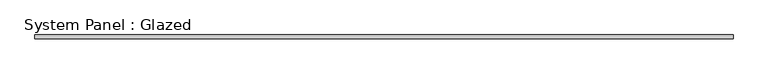
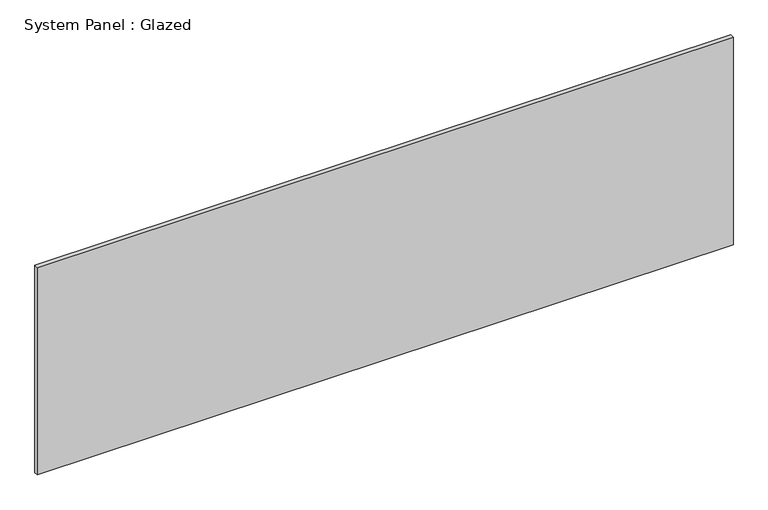
"""IFC4 building model written with IfcOpenShell, lengths in millimetres: plate geometry, System Panel : Glazed."""

from ifc_helpers import new_model, si_unit, origin, origin_with_axes, place, context, project, spatial, polyline, outline, extrude, source, transform, mapped, element, save


def system_panel_glazed_648d5b1a(model_context):
    return source(origin(), model_context, "Body", "SweptSolid", [
        extrude(outline(polyline([(2317.75, 19.05), (-2317.75, 19.05), (-2317.75, 44.45), (2317.75, 44.45), (2317.75, 19.05)])), origin_with_axes(), (0.0, 0.0, 1.0), 1460.5),
    ])


if __name__ == "__main__":
    model = new_model("IFC4")
    model_context = context("Model", 3, world=origin())
    ifc_project = project(units=[si_unit("LENGTHUNIT", "METRE", prefix="MILLI")], contexts=[model_context])
    site = spatial("IfcSite", under=ifc_project)
    building = spatial("IfcBuilding", under=site)
    placement = place(None, origin())
    system_panel_glazed_shape = system_panel_glazed_648d5b1a(model_context)
    element("IfcPlate", 1, ObjectType="System Panel : Glazed", at=placement, inside=building, context=model_context, shape_type="MappedRepresentation", body=[
        mapped(system_panel_glazed_shape, transform((0.0, 0.0, 0.0), x_axis=(1.0, 0.0, 0.0), y_axis=(0.0, 1.0, 0.0), z_axis=(0.0, 0.0, 1.0))),
    ])
    save(model, "model.ifc")

# Revit data of these elements
# Type "System Panel : Glazed"
#   Construction Type Id = "GSP4R"
#   Analytic Construction = "1/8 in Pilkington single glazing"
#   Visual Light Transmittance = 0.9
#   Solar Heat Gain Coefficient = 0.86
#   Heat Transfer Coefficient (U) = 1.18115 BTU/(h·ft²·°F)
# Element 1 (IfcPlate, "System Panel : Glazed")
#   Materials on its faces: "Glass"
# Materials
#   "Glass": class "Glass", colour RGB 0 128 192, transparency 0.75, Description = "Soda Lime Glass", Cost = 0
